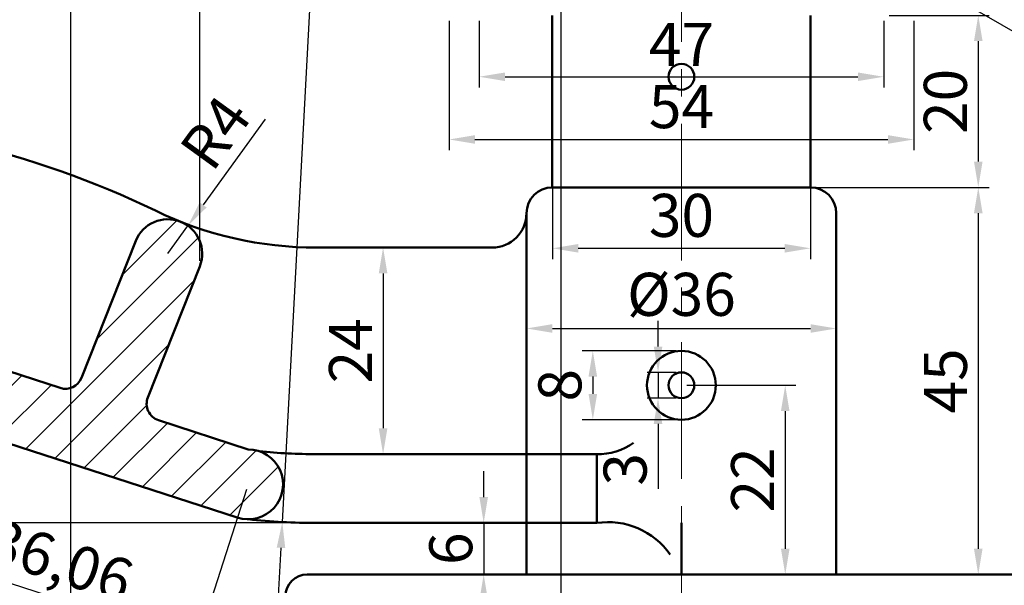
# Model space of a CAD drawing. Units: millimetres. Extents: x 98 to 674, y 38 to 476.
# Tile 3 of 7: x 200 to 315, y 131 to 197. Entities that reach past the tile are written whole.
import ezdxf

# ---------------------------------------------------------------- set-up
doc = ezdxf.new("R2010")
doc.units = ezdxf.units.MM
doc.header["$LTSCALE"] = 0.5
doc.linetypes.add('CENTER', pattern=[50.8, 31.75, -6.35, 6.35, -6.35])
for name, color, linetype, lineweight in [('M-CNTR', 1, 'CENTER', 18), ('M-DIMS', 2, 'Continuous', 25), ('M-HATC', 8, 'Continuous', 18), ('M-OUTL', 7, 'Continuous', 50)]:
    doc.layers.add(name, color=color, linetype=linetype, lineweight=lineweight)
doc.styles.get("Standard").update_dxf_attribs({"font": 'arial.ttf'})
doc.dimstyles.new('ISO-25', dxfattribs={"dimtxt": 5, "dimasz": 3, "dimexe": 1.25, "dimexo": 0.625, "dimtad": 1, "dimtxsty": 'Standard', "dimcen": 2.5, "dimadec": 0, "dimazin": 0, "dimtfac": 1, "dimtmove": 0, "dimatfit": 3, "dimfxl": 1, "dimarcsym": 0})

# ---------------------------------------------------------------- blocks, each defined once
blk = doc.blocks.new('*D21')
at = {"layer": 'Defpoints', "color": 0, "ltscale": 0.5, "transparency": 16777216}
for p in [(327.04, 262.55), (348.82, 249.98), (295.37, 207.69)]:
    blk.add_point(p, dxfattribs=at)
at = {"layer": 'M-DIMS', "color": 0, "lineweight": -2, "ltscale": 0.5, "transparency": 16777216}
for p, q in [((327.58, 262.24), (349.9, 249.35)), ((318.64, 197.71), (347.32, 247.38)), ((295.91, 207.37), (318.22, 194.49))]:
    blk.add_line(p, q, dxfattribs=at)
at = {"layer": 'M-DIMS', "color": 0, "ltscale": 0.5, "transparency": 16777216}
for points in [[(346.89, 247.63), (347.75, 247.13), (348.82, 249.98)], [(318.21, 197.96), (319.08, 197.46), (317.14, 195.11)]]:
    blk.add_solid(points, dxfattribs=at)
at = {"layer": 'M-DIMS', "color": 0, "ltscale": 0.5, "transparency": 16777216, "insert": (329.84, 224.36), "char_height": 5, "attachment_point": 5, "rotation": 60}
blk.add_mtext('63,35', dxfattribs=at)
blk = doc.blocks.new('*D29')
at = {"layer": 'Defpoints', "color": 0, "ltscale": 0.5, "transparency": 16777216}
for p in [(253.87, 197.69), (300.87, 197.69), (300.87, 190.55)]:
    blk.add_point(p, dxfattribs=at)
at = {"layer": 'M-DIMS', "color": 0, "lineweight": -2, "ltscale": 0.5, "transparency": 16777216}
for p, q in [((253.87, 197.06), (253.87, 189.3)), ((300.87, 197.06), (300.87, 189.3)), ((256.87, 190.55), (297.87, 190.55))]:
    blk.add_line(p, q, dxfattribs=at)
at = {"layer": 'M-DIMS', "color": 0, "ltscale": 0.5, "transparency": 16777216}
for points in [[(256.87, 191.05), (256.87, 190.05), (253.87, 190.55)], [(297.87, 191.05), (297.87, 190.05), (300.87, 190.55)]]:
    blk.add_solid(points, dxfattribs=at)
at = {"layer": 'M-DIMS', "color": 0, "ltscale": 0.5, "transparency": 16777216, "insert": (277.37, 193.67), "char_height": 5, "attachment_point": 5}
blk.add_mtext('47', dxfattribs=at)
blk = doc.blocks.new('*D30')
at = {"layer": 'Defpoints', "color": 0, "ltscale": 0.5, "transparency": 16777216}
for p in [(250.37, 197.69), (304.37, 197.69), (304.37, 183.26)]:
    blk.add_point(p, dxfattribs=at)
at = {"layer": 'M-DIMS', "color": 0, "lineweight": -2, "ltscale": 0.5, "transparency": 16777216}
for p, q in [((250.37, 197.06), (250.37, 182.01)), ((304.37, 197.06), (304.37, 182.01)), ((253.37, 183.26), (301.37, 183.26))]:
    blk.add_line(p, q, dxfattribs=at)
at = {"layer": 'M-DIMS', "color": 0, "ltscale": 0.5, "transparency": 16777216}
for points in [[(253.37, 183.76), (253.37, 182.76), (250.37, 183.26)], [(301.37, 183.76), (301.37, 182.76), (304.37, 183.26)]]:
    blk.add_solid(points, dxfattribs=at)
at = {"layer": 'M-DIMS', "color": 0, "ltscale": 0.5, "transparency": 16777216, "insert": (277.37, 186.43), "char_height": 5, "attachment_point": 5}
blk.add_mtext('54', dxfattribs=at)
blk = doc.blocks.new('*D31')
at = {"layer": 'Defpoints', "color": 0, "ltscale": 0.5, "transparency": 16777216}
for p in [(262.37, 179.48), (292.37, 179.48), (292.37, 170.61)]:
    blk.add_point(p, dxfattribs=at)
at = {"layer": 'M-DIMS', "color": 0, "lineweight": -2, "ltscale": 0.5, "transparency": 16777216}
for p, q in [((262.37, 178.85), (262.37, 169.36)), ((292.37, 178.85), (292.37, 169.36)), ((265.37, 170.61), (289.37, 170.61))]:
    blk.add_line(p, q, dxfattribs=at)
at = {"layer": 'M-DIMS', "color": 0, "ltscale": 0.5, "transparency": 16777216}
for points in [[(265.37, 171.11), (265.37, 170.11), (262.37, 170.61)], [(289.37, 171.11), (289.37, 170.11), (292.37, 170.61)]]:
    blk.add_solid(points, dxfattribs=at)
at = {"layer": 'M-DIMS', "color": 0, "ltscale": 0.5, "transparency": 16777216, "insert": (277.37, 173.79), "char_height": 5, "attachment_point": 5}
blk.add_mtext('30', dxfattribs=at)
blk = doc.blocks.new('*D32')
at = {"layer": 'Defpoints', "color": 0, "ltscale": 0.5, "transparency": 16777216}
for p in [(259.37, 161.17), (295.37, 161.29), (295.37, 161.17)]:
    blk.add_point(p, dxfattribs=at)
at = {"layer": 'M-DIMS', "color": 0, "lineweight": -2, "ltscale": 0.5, "transparency": 16777216}
for p, q in [((259.37, 161.79), (259.37, 162.54)), ((295.37, 161.79), (295.37, 162.54)), ((262.37, 161.29), (292.37, 161.29))]:
    blk.add_line(p, q, dxfattribs=at)
at = {"layer": 'M-DIMS', "color": 0, "ltscale": 0.5, "transparency": 16777216}
for points in [[(262.37, 161.79), (262.37, 160.79), (259.37, 161.29)], [(292.37, 161.79), (292.37, 160.79), (295.37, 161.29)]]:
    blk.add_solid(points, dxfattribs=at)
at = {"layer": 'M-DIMS', "color": 0, "ltscale": 0.5, "transparency": 16777216, "insert": (277.37, 164.61), "char_height": 5, "attachment_point": 5}
blk.add_mtext('%%C36', dxfattribs=at)
blk = doc.blocks.new('*D33')
at = {"layer": 'Defpoints', "color": 0, "ltscale": 0.5, "transparency": 16777216}
for p in [(300.87, 197.69), (292.37, 177.69), (311.86, 177.69)]:
    blk.add_point(p, dxfattribs=at)
at = {"layer": 'M-DIMS', "color": 0, "lineweight": -2, "ltscale": 0.5, "transparency": 16777216}
for p, q in [((301.49, 197.69), (313.11, 197.69)), ((311.86, 194.69), (311.86, 180.69)), ((292.99, 177.69), (313.11, 177.69))]:
    blk.add_line(p, q, dxfattribs=at)
at = {"layer": 'M-DIMS', "color": 0, "ltscale": 0.5, "transparency": 16777216}
for points in [[(311.36, 194.69), (312.36, 194.69), (311.86, 197.69)], [(311.36, 180.69), (312.36, 180.69), (311.86, 177.69)]]:
    blk.add_solid(points, dxfattribs=at)
at = {"layer": 'M-DIMS', "color": 0, "ltscale": 0.5, "transparency": 16777216, "insert": (308.68, 187.69), "char_height": 5, "attachment_point": 5, "rotation": 90}
blk.add_mtext('20', dxfattribs=at)
blk = doc.blocks.new('*D34')
at = {"layer": 'Defpoints', "color": 0, "ltscale": 0.5, "transparency": 16777216}
for p in [(303.05, 177.69), (303.05, 132.69), (311.86, 132.69)]:
    blk.add_point(p, dxfattribs=at)
at = {"layer": 'M-DIMS', "color": 0, "lineweight": -2, "ltscale": 0.5, "transparency": 16777216}
for p, q in [((303.68, 177.69), (313.11, 177.69)), ((311.86, 174.69), (311.86, 135.69)), ((303.68, 132.69), (313.11, 132.69))]:
    blk.add_line(p, q, dxfattribs=at)
at = {"layer": 'M-DIMS', "color": 0, "ltscale": 0.5, "transparency": 16777216}
for points in [[(311.36, 174.69), (312.36, 174.69), (311.86, 177.69)], [(311.36, 135.69), (312.36, 135.69), (311.86, 132.69)]]:
    blk.add_solid(points, dxfattribs=at)
at = {"layer": 'M-DIMS', "color": 0, "ltscale": 0.5, "transparency": 16777216, "insert": (308.69, 155.19), "char_height": 5, "attachment_point": 5, "rotation": 90}
blk.add_mtext('45', dxfattribs=at)
blk = doc.blocks.new('*D35')
at = {"layer": 'Defpoints', "color": 0, "ltscale": 0.5, "transparency": 16777216}
for p in [(277.37, 154.69), (277.37, 132.69), (289.43, 132.69)]:
    blk.add_point(p, dxfattribs=at)
at = {"layer": 'M-DIMS', "color": 0, "lineweight": -2, "ltscale": 0.5, "transparency": 16777216}
for p, q in [((277.99, 154.69), (290.68, 154.69)), ((289.43, 151.69), (289.43, 135.69)), ((277.99, 132.69), (290.68, 132.69))]:
    blk.add_line(p, q, dxfattribs=at)
at = {"layer": 'M-DIMS', "color": 0, "ltscale": 0.5, "transparency": 16777216}
for points in [[(288.93, 151.69), (289.93, 151.69), (289.43, 154.69)], [(288.93, 135.69), (289.93, 135.69), (289.43, 132.69)]]:
    blk.add_solid(points, dxfattribs=at)
at = {"layer": 'M-DIMS', "color": 0, "ltscale": 0.5, "transparency": 16777216, "insert": (286.29, 143.69), "char_height": 5, "attachment_point": 5, "rotation": 90}
blk.add_mtext('22', dxfattribs=at)
blk = doc.blocks.new('*D36')
at = {"layer": 'Defpoints', "color": 0, "ltscale": 0.5, "transparency": 16777216}
for p in [(277.37, 156.19), (274.65, 153.19), (277.37, 153.19)]:
    blk.add_point(p, dxfattribs=at)
at = {"layer": 'M-DIMS', "color": 0, "lineweight": -2, "ltscale": 0.5, "transparency": 16777216}
for p, q in [((274.65, 159.19), (274.65, 162.19)), ((276.74, 156.19), (273.4, 156.19)), ((274.65, 156.19), (274.65, 153.19)), ((276.74, 153.19), (273.4, 153.19)), ((274.65, 150.19), (274.65, 142.66))]:
    blk.add_line(p, q, dxfattribs=at)
at = {"layer": 'M-DIMS', "color": 0, "ltscale": 0.5, "transparency": 16777216}
for points in [[(274.15, 159.19), (275.15, 159.19), (274.65, 156.19)], [(274.15, 150.19), (275.15, 150.19), (274.65, 153.19)]]:
    blk.add_solid(points, dxfattribs=at)
at = {"layer": 'M-DIMS', "color": 0, "ltscale": 0.5, "transparency": 16777216, "insert": (271.47, 144.92), "char_height": 5, "attachment_point": 5, "rotation": 90}
blk.add_mtext('3', dxfattribs=at)
blk = doc.blocks.new('*D37')
at = {"layer": 'Defpoints', "color": 0, "ltscale": 0.5, "transparency": 16777216}
for p in [(277.37, 158.69), (267.07, 150.69), (277.37, 150.69)]:
    blk.add_point(p, dxfattribs=at)
at = {"layer": 'M-DIMS', "color": 0, "lineweight": -2, "ltscale": 0.5, "transparency": 16777216}
for p, q in [((276.74, 158.69), (265.82, 158.69)), ((267.07, 155.69), (267.07, 153.69)), ((276.74, 150.69), (265.82, 150.69))]:
    blk.add_line(p, q, dxfattribs=at)
at = {"layer": 'M-DIMS', "color": 0, "ltscale": 0.5, "transparency": 16777216}
for points in [[(266.57, 155.69), (267.57, 155.69), (267.07, 158.69)], [(266.57, 153.69), (267.57, 153.69), (267.07, 150.69)]]:
    blk.add_solid(points, dxfattribs=at)
at = {"layer": 'M-DIMS', "color": 0, "ltscale": 0.5, "transparency": 16777216, "insert": (263.89, 154.69), "char_height": 5, "attachment_point": 5, "rotation": 90}
blk.add_mtext('8', dxfattribs=at)
blk = doc.blocks.new('*D38')
at = {"layer": 'Defpoints', "color": 0, "ltscale": 0.5, "transparency": 16777216}
for p in [(254.39, 138.69), (254.39, 132.69), (254.39, 132.69)]:
    blk.add_point(p, dxfattribs=at)
at = {"layer": 'M-DIMS', "color": 0, "lineweight": -2, "ltscale": 0.5, "transparency": 16777216}
for p, q in [((254.39, 141.69), (254.39, 144.69)), ((254.39, 138.69), (254.39, 132.69)), ((255.02, 138.69), (255.64, 138.69)), ((255.02, 132.69), (255.64, 132.69)), ((254.39, 129.69), (254.39, 126.69))]:
    blk.add_line(p, q, dxfattribs=at)
at = {"layer": 'M-DIMS', "color": 0, "ltscale": 0.5, "transparency": 16777216}
for points in [[(253.89, 141.69), (254.89, 141.69), (254.39, 138.69)], [(253.89, 129.69), (254.89, 129.69), (254.39, 132.69)]]:
    blk.add_solid(points, dxfattribs=at)
at = {"layer": 'M-DIMS', "color": 0, "ltscale": 0.5, "transparency": 16777216, "insert": (251.21, 135.69), "char_height": 5, "attachment_point": 5, "rotation": 90}
blk.add_mtext('6', dxfattribs=at)
blk = doc.blocks.new('*D50')
at = {"layer": 'Defpoints', "color": 0, "ltscale": 0.5, "transparency": 16777216}
for p in [(149.37, 153.69), (149.37, 113.28), (277.37, 112.69)]:
    blk.add_point(p, dxfattribs=at)
at = {"layer": 'M-DIMS', "color": 0, "lineweight": -2, "ltscale": 0.5, "transparency": 16777216}
for p, q in [((149.37, 153.06), (149.37, 112.03)), ((277.37, 113.31), (277.37, 114.53)), ((274.37, 113.28), (152.37, 113.28))]:
    blk.add_line(p, q, dxfattribs=at)
at = {"layer": 'M-DIMS', "color": 0, "ltscale": 0.5, "transparency": 16777216}
for points in [[(152.37, 113.78), (152.37, 112.78), (149.37, 113.28)], [(274.37, 113.78), (274.37, 112.78), (277.37, 113.28)]]:
    blk.add_solid(points, dxfattribs=at)
at = {"layer": 'M-DIMS', "color": 0, "ltscale": 0.5, "transparency": 16777216, "insert": (213.37, 116.46), "char_height": 5, "attachment_point": 5}
blk.add_mtext('128', dxfattribs=at)
blk = doc.blocks.new('*D52')
at = {"layer": 'Defpoints', "color": 0, "ltscale": 0.5, "transparency": 16777216}
for p in [(135.65, 153.69), (149.37, 153.69), (251.25, 138.69)]:
    blk.add_point(p, dxfattribs=at)
at = {"layer": 'M-DIMS', "color": 0, "lineweight": -2, "ltscale": 0.5, "transparency": 16777216}
for p, q in [((148.74, 153.69), (134.4, 153.69)), ((135.65, 141.69), (135.65, 150.69)), ((250.63, 138.69), (134.4, 138.69))]:
    blk.add_line(p, q, dxfattribs=at)
at = {"layer": 'M-DIMS', "color": 0, "ltscale": 0.5, "transparency": 16777216}
for points in [[(135.15, 150.69), (136.15, 150.69), (135.65, 153.69)], [(135.15, 141.69), (136.15, 141.69), (135.65, 138.69)]]:
    blk.add_solid(points, dxfattribs=at)
at = {"layer": 'M-DIMS', "color": 0, "ltscale": 0.5, "transparency": 16777216, "insert": (132.47, 146.19), "char_height": 5, "attachment_point": 5, "rotation": 90}
blk.add_mtext('15', dxfattribs=at)
blk = doc.blocks.new('*D53')
at = {"layer": 'Defpoints', "color": 0, "ltscale": 0.5, "transparency": 16777216}
for p in [(192.69, 154.23), (227.02, 143.17), (221.06, 124.69)]:
    blk.add_point(p, dxfattribs=at)
at = {"layer": 'M-DIMS', "color": 0, "lineweight": -2, "ltscale": 0.5, "transparency": 16777216}
for p, q in [((192.5, 153.64), (186.35, 134.56)), ((226.82, 142.58), (220.68, 123.5)), ((189.59, 134.83), (218.21, 125.61))]:
    blk.add_line(p, q, dxfattribs=at)
at = {"layer": 'M-DIMS', "color": 0, "ltscale": 0.5, "transparency": 16777216}
for points in [[(189.75, 135.31), (189.44, 134.36), (186.74, 135.75)], [(218.36, 126.09), (218.05, 125.14), (221.06, 124.69)]]:
    blk.add_solid(points, dxfattribs=at)
at = {"layer": 'M-DIMS', "color": 0, "ltscale": 0.5, "transparency": 16777216, "insert": (205.01, 133.68), "char_height": 5, "attachment_point": 5, "rotation": 342.137}
blk.add_mtext('36,06', dxfattribs=at)
blk = doc.blocks.new('*D54')
at = {"layer": 'Defpoints', "color": 0, "ltscale": 0.5, "transparency": 16777216}
for p in [(245.17, 170.69), (242.7, 146.69), (245.17, 146.69)]:
    blk.add_point(p, dxfattribs=at)
at = {"layer": 'M-DIMS', "color": 0, "lineweight": -2, "ltscale": 0.5, "transparency": 16777216}
for p, q in [((244.55, 170.69), (241.45, 170.69)), ((242.7, 167.69), (242.7, 149.69)), ((244.55, 146.69), (241.45, 146.69))]:
    blk.add_line(p, q, dxfattribs=at)
at = {"layer": 'M-DIMS', "color": 0, "ltscale": 0.5, "transparency": 16777216}
for points in [[(242.2, 167.69), (243.2, 167.69), (242.7, 170.69)], [(242.2, 149.69), (243.2, 149.69), (242.7, 146.69)]]:
    blk.add_solid(points, dxfattribs=at)
at = {"layer": 'M-DIMS', "color": 0, "ltscale": 0.5, "transparency": 16777216, "insert": (239.56, 158.69), "char_height": 5, "attachment_point": 5, "rotation": 90}
blk.add_mtext('24', dxfattribs=at)
blk = doc.blocks.new('*D68')
at = {"layer": 'Defpoints', "color": 0, "ltscale": 0.5, "transparency": 16777216}
for p in [(263.37, 325.69), (206.37, 226.96), (263.37, 42.76)]:
    blk.add_point(p, dxfattribs=at)
at = {"layer": 'M-DIMS', "color": 0, "lineweight": -2, "ltscale": 0.5, "transparency": 16777216}
for p, q in [((263.37, 325.06), (263.37, 41.51)), ((206.37, 226.33), (206.37, 41.51)), ((209.37, 42.76), (260.37, 42.76))]:
    blk.add_line(p, q, dxfattribs=at)
at = {"layer": 'M-DIMS', "color": 0, "ltscale": 0.5, "transparency": 16777216}
for points in [[(209.37, 43.26), (209.37, 42.26), (206.37, 42.76)], [(260.37, 43.26), (260.37, 42.26), (263.37, 42.76)]]:
    blk.add_solid(points, dxfattribs=at)
at = {"layer": 'M-DIMS', "color": 0, "ltscale": 0.5, "transparency": 16777216, "insert": (234.87, 45.93), "char_height": 5, "attachment_point": 5}
blk.add_mtext('57', dxfattribs=at)
blk = doc.blocks.new('*D71')
at = {"layer": 'Defpoints', "color": 0, "ltscale": 0.5, "transparency": 16777216}
for p in [(269.37, 413.69), (121.37, 76.69), (269.37, 76.69)]:
    blk.add_point(p, dxfattribs=at)
at = {"layer": 'M-DIMS', "color": 0, "lineweight": -2, "ltscale": 0.5, "transparency": 16777216}
for p, q in [((268.74, 413.69), (120.12, 413.69)), ((121.37, 410.69), (121.37, 79.69)), ((268.74, 76.69), (120.12, 76.69))]:
    blk.add_line(p, q, dxfattribs=at)
at = {"layer": 'M-DIMS', "color": 0, "ltscale": 0.5, "transparency": 16777216}
for points in [[(120.87, 410.69), (121.87, 410.69), (121.37, 413.69)], [(120.87, 79.69), (121.87, 79.69), (121.37, 76.69)]]:
    blk.add_solid(points, dxfattribs=at)
at = {"layer": 'M-DIMS', "color": 0, "ltscale": 0.5, "transparency": 16777216, "insert": (118.19, 245.19), "char_height": 5, "attachment_point": 5, "rotation": 90}
blk.add_mtext('337', dxfattribs=at)
blk = doc.blocks.new('*D72')
at = {"layer": 'Defpoints', "color": 0, "ltscale": 0.5, "transparency": 16777216}
for p in [(149.37, 196.69), (323.37, 130.19), (323.37, 42.76)]:
    blk.add_point(p, dxfattribs=at)
at = {"layer": 'M-DIMS', "color": 0, "lineweight": -2, "ltscale": 0.5, "transparency": 16777216}
for p, q in [((149.37, 196.06), (149.37, 41.51)), ((323.37, 129.56), (323.37, 41.51)), ((152.37, 42.76), (320.37, 42.76))]:
    blk.add_line(p, q, dxfattribs=at)
at = {"layer": 'M-DIMS', "color": 0, "ltscale": 0.5, "transparency": 16777216}
for points in [[(152.37, 43.26), (152.37, 42.26), (149.37, 42.76)], [(320.37, 43.26), (320.37, 42.26), (323.37, 42.76)]]:
    blk.add_solid(points, dxfattribs=at)
at = {"layer": 'M-DIMS', "color": 0, "ltscale": 0.5, "transparency": 16777216, "insert": (236.37, 45.9), "char_height": 5, "attachment_point": 5}
blk.add_mtext('174', dxfattribs=at)
blk = doc.blocks.new('*D73')
at = {"layer": 'Defpoints', "color": 0, "ltscale": 0.5, "transparency": 16777216}
for p in [(221.4, 441.69), (221.4, 168.51), (149.37, 153.69)]:
    blk.add_point(p, dxfattribs=at)
at = {"layer": 'M-DIMS', "color": 0, "lineweight": -2, "ltscale": 0.5, "transparency": 16777216}
for p, q in [((149.37, 154.31), (149.37, 442.94)), ((221.4, 169.14), (221.4, 442.94)), ((152.37, 441.69), (218.4, 441.69))]:
    blk.add_line(p, q, dxfattribs=at)
at = {"layer": 'M-DIMS', "color": 0, "ltscale": 0.5, "transparency": 16777216}
for points in [[(152.37, 442.19), (152.37, 441.19), (149.37, 441.69)], [(218.4, 442.19), (218.4, 441.19), (221.4, 441.69)]]:
    blk.add_solid(points, dxfattribs=at)
at = {"layer": 'M-DIMS', "color": 0, "ltscale": 0.5, "transparency": 16777216, "insert": (185.38, 444.87), "char_height": 5, "attachment_point": 5}
blk.add_mtext('72.03', dxfattribs=at)
blk = doc.blocks.new('*D74')
at = {"layer": 'Defpoints', "color": 0, "ltscale": 0.5, "transparency": 16777216}
for p in [(220.03, 173.23), (217.68, 169.99)]:
    blk.add_point(p, dxfattribs=at)
at = {"layer": 'M-DIMS', "color": 0, "lineweight": -2, "ltscale": 0.5, "transparency": 16777216}
for p, q in [((228.99, 185.61), (221.79, 175.66)), ((217.68, 169.99), (220.03, 173.23))]:
    blk.add_line(p, q, dxfattribs=at)
at = {"layer": 'M-DIMS', "color": 0, "ltscale": 0.5, "transparency": 16777216}
blk.add_solid([(221.38, 175.95), (222.19, 175.36), (220.03, 173.23)], dxfattribs=at)
at = {"layer": 'M-DIMS', "color": 0, "ltscale": 0.5, "transparency": 16777216, "insert": (223.74, 183.68), "char_height": 5, "attachment_point": 5, "rotation": 54.0979}
blk.add_mtext('R4', dxfattribs=at)
blk = doc.blocks.new('*D76')
at = {"layer": 'Defpoints', "color": 0, "ltscale": 0.5, "transparency": 16777216}
for p in [(234.98, 213.69), (230.99, 138.79)]:
    blk.add_point(p, dxfattribs=at)
at = {"layer": 'M-DIMS', "color": 0, "lineweight": -2, "ltscale": 0.5, "transparency": 16777216}
for p, q in [((234.98, 213.69), (230.99, 138.79)), ((228.25, 87.25), (230.84, 135.8))]:
    blk.add_line(p, q, dxfattribs=at)
at = {"layer": 'M-DIMS', "color": 0, "ltscale": 0.5, "transparency": 16777216}
blk.add_solid([(230.34, 135.82), (231.33, 135.77), (230.99, 138.79)], dxfattribs=at)
at = {"layer": 'M-DIMS', "color": 0, "ltscale": 0.5, "transparency": 16777216, "insert": (225.44, 94.02), "char_height": 5, "attachment_point": 5, "rotation": 86.9505}
blk.add_mtext('R75', dxfattribs=at)
blk = doc.blocks.new('*D78')
at = {"layer": 'Defpoints', "color": 0, "ltscale": 0.5, "transparency": 16777216}
for p in [(291.37, 325.69), (348.37, 226.96)]:
    blk.add_point(p, dxfattribs=at)
at = {"layer": 'M-DIMS', "color": 0, "lineweight": -2, "ltscale": 0.5, "transparency": 16777216}
for p, q in [((291.37, 325.69), (348.37, 226.96)), ((386.83, 160.33), (349.87, 224.36))]:
    blk.add_line(p, q, dxfattribs=at)
at = {"layer": 'M-DIMS', "color": 0, "ltscale": 0.5, "transparency": 16777216}
blk.add_solid([(350.3, 224.61), (349.43, 224.11), (348.37, 226.96)], dxfattribs=at)
at = {"layer": 'M-DIMS', "color": 0, "ltscale": 0.5, "transparency": 16777216, "insert": (385.28, 169.29), "char_height": 5, "attachment_point": 5, "rotation": 300.0001}
blk.add_mtext('R114', dxfattribs=at)

msp = doc.modelspace()

# ---------------------------------------------------------------- hatches: boundary and pattern name
at = {"layer": 'M-HATC', "ltscale": 0.5}
h = msp.add_hatch(dxfattribs=at)
h.set_pattern_fill('ANSI31', color=256)
h.paths.add_polyline_path([(215.3645, 153.2734), (221.3997, 168.5142, 1), (213.9617, 171.4596), (207.6565, 155.5371, -0.39645231), (205.1754, 154.3725), (194.5293, 157.8537, 1), (190.8572, 150.6104, -0.00464805), (192.1907, 150.2028), (225.763, 139.3083, 1.17062936), (227.0163, 147.2309), (216.6024, 150.6361, -0.43220072)])

# ---------------------------------------------------------------- linework, layer by layer
at = {"layer": 'M-CNTR'}
msp.add_line((277.365, 413.6855), (277.365, 70.7639), dxfattribs=at)
at = {"layer": 'M-OUTL'}
for p, q in [((262.365, 197.6855), (262.365, 177.6855)), ((292.365, 177.6855), (292.365, 197.6855)), ((262.365, 177.6855), (292.365, 177.6855)), ((262.365, 177.6855), (292.365, 177.6855)), ((259.365, 132.6855), (259.365, 174.6855)), ((295.365, 174.6855), (295.365, 132.6855)), ((267.5202, 146.6855), (234.9849, 146.6855)), ((267.5202, 138.6855), (234.9849, 138.6855)), ((295.365, 132.6855), (259.365, 132.6855))]:
    msp.add_line(p, q, dxfattribs=at)
at = {"layer": 'M-OUTL', "ltscale": 0.5}
for p, q in [((207.6565, 155.5371), (213.9617, 171.4596)), ((215.3645, 153.2734), (221.3997, 168.5142)), ((194.5293, 157.8537), (205.1754, 154.3725)), ((192.1907, 150.2028), (225.763, 139.3083)), ((216.6024, 150.6361), (227.0163, 147.2309)), ((267.5202, 146.6855), (267.5202, 138.6855)), ((277.365, 132.6855), (277.365, 138.6855))]:
    msp.add_line(p, q, dxfattribs=at)
at = {"layer": 'M-OUTL'}
msp.add_lwpolyline([(259.365, 174.6855), (259.365, 174.6855, -0.41421356), (255.365, 170.6855), (234.9849, 170.6855, -0.11323701), (216.2416, 174.9855, 0.11151094), (170.3309, 185.683, -0.41221797), (165.365, 190.6829), (165.365, 196.6855)], format="xyb", dxfattribs=at)
msp.add_lwpolyline([(320.865, 132.6855), (233.865, 132.6855, 1), (233.865, 127.6855), (320.865, 127.6855, 1)], format="xyb", close=True, dxfattribs=at)
at = {"layer": 'M-OUTL', "ltscale": 0.5}
msp.add_circle((277.365, 190.5497), 1.5, dxfattribs=at)
at = {"layer": 'M-OUTL'}
for radius in [4, 1.5]:
    msp.add_circle((277.365, 154.6855), radius, dxfattribs=at)
for centre, radius, start, end in [((262.365, 174.6855), 3, 90, 180), ((292.365, 174.6855), 3, 0, 90), ((234.9849, 213.6855), 67, 264.284271, 270), ((234.9849, 213.6855), 75, 263.900929, 270)]:
    msp.add_arc(centre, radius, start, end, dxfattribs=at)
at = {"layer": 'M-OUTL', "ltscale": 0.5}
for centre, radius, start, end in [((217.6807, 169.9869), 4, 338.396932, 158.396932), ((205.797, 156.2735), 2, 251.893074, 338.396932), ((217.224, 152.537), 2, 158.396932, 251.893074), ((267.6667, 153.9397), 7.2557, 268.843493, 304.869517), ((227.0163, 143.1705), 4.0605, 252.021289, 90), ((268.8247, 129.959), 8.8234, 34.895768, 98.502029)]:
    msp.add_arc(centre, radius, start, end, dxfattribs=at)

# ---------------------------------------------------------------- dimensions: what is measured, and where the dimension line sits
at = {"layer": 'M-DIMS', "ltscale": 0.5}
for base, p1, p2, override, picture, middle in [((221.3997, 441.6855), (149.365, 153.6855), (221.3997, 168.5142), {"dimdec": 2, "dimlfac": 1, "dimrnd": 0, "dimzin": 0, "dimdsep": 46, "dimlunit": 2}, '*D73', (185.3824, 444.8651)), ((263.365, 42.7639), (206.365, 226.9586), (263.365, 325.6855), {"dimdec": 0, "dimlfac": 1, "dimrnd": 0, "dimzin": 0, "dimdsep": 46, "dimlunit": 2}, '*D68', (234.865, 45.9316)), ((304.365, 183.2593), (250.365, 197.6855), (304.365, 197.6855), {"dimclrd": 0, "dimclre": 0, "dimclrt": 0}, '*D30', (277.365, 186.4269)), ((300.865, 190.5497), (253.865, 197.6855), (300.865, 197.6855), {"dimclrd": 0, "dimclre": 0, "dimclrt": 0}, '*D29', (277.365, 193.6747)), ((323.365, 42.7639), (149.365, 196.6855), (323.365, 130.1855), {"dimdec": 0, "dimlfac": 1, "dimrnd": 0, "dimzin": 0, "dimdsep": 46, "dimlunit": 2}, '*D72', (236.365, 45.8992)), ((292.365, 170.6148), (262.365, 179.4762), (292.365, 179.4762), {"dimclrd": 0, "dimclre": 0, "dimclrt": 0}, '*D31', (277.365, 173.7944)), ((149.365, 113.2817), (277.365, 112.6855), (149.365, 153.6855), {"dimclrd": 0, "dimclre": 0, "dimclrt": 0}, '*D50', (213.365, 116.4596))]:
    dim = msp.add_linear_dim(base=base, p1=p1, p2=p2, dimstyle='ISO-25', override=override, dxfattribs=at)
    dim.commit()
    dim.dimension.update_dxf_attribs({"geometry": picture, "text_midpoint": middle})
for base, p1, p2, override, picture, middle in [((121.365, 76.6855), (269.365, 413.6855), (269.365, 76.6855), {"dimdec": 0, "dimlfac": 1, "dimrnd": 0, "dimzin": 0, "dimdsep": 46, "dimlunit": 2}, '*D71', (118.1855, 245.1855)), ((311.8607, 177.6855), (300.865, 197.6855), (292.365, 177.6855), {"dimclrd": 0, "dimclre": 0, "dimclrt": 0}, '*D33', (308.6828, 187.6855)), ((311.8607, 132.6855), (303.0504, 177.6855), (303.0504, 132.6855), {"dimclrd": 0, "dimclre": 0, "dimclrt": 0}, '*D34', (308.6931, 155.1855)), ((274.6545, 153.1855), (277.365, 156.1855), (277.365, 153.1855), {"dimclrd": 0, "dimclre": 0, "dimclrt": 0}, '*D36', (271.475, 144.9234)), ((267.0703, 150.6855), (277.365, 158.6855), (277.365, 150.6855), {"dimclrd": 0, "dimclre": 0, "dimclrt": 0}, '*D37', (263.8924, 154.6855)), ((289.426, 132.6855), (277.365, 154.6855), (277.365, 132.6855), {"dimclrd": 0, "dimclre": 0, "dimclrt": 0}, '*D35', (286.2908, 143.6855)), ((135.6524, 153.6855), (251.2525, 138.6855), (149.365, 153.6855), {"dimclrd": 0, "dimclre": 0, "dimclrt": 0}, '*D52', (132.4745, 146.1855)), ((254.3923, 132.6855), (254.3923, 138.6855), (254.3923, 132.6855), {"dimclrd": 0, "dimclre": 0, "dimclrt": 0}, '*D38', (251.2145, 135.6855))]:
    dim = msp.add_linear_dim(base=base, p1=p1, p2=p2, angle=90, dimstyle='ISO-25', override=override, dxfattribs=at)
    dim.commit()
    dim.dimension.update_dxf_attribs({"geometry": picture, "text_midpoint": middle})
for center, mpoint, picture, middle in [((291.365, 325.6855), (348.3652, 226.9587), '*D78', (382.5653, 167.7226)), ((234.9849, 213.6855), (230.995, 138.7917), '*D76', (228.601, 93.8554))]:
    dim = msp.add_radius_dim(center=center, mpoint=mpoint, dimstyle='ISO-25', override={"dimdec": 0, "dimlfac": 1, "dimrnd": 0, "dimzin": 0, "dimdsep": 46, "dimlunit": 2}, dxfattribs=at)
    dim.commit()
    dim.dimension.update_dxf_attribs({"geometry": picture, "text_midpoint": middle, "dimtype": 164})
for p1, p2, distance, picture, middle in [((295.365, 207.6855), (327.0419, 262.5515), -25.146, '*D21', (329.8371, 224.3604)), ((245.175, 170.6855), (245.175, 146.6855), -2.4781, '*D54', (239.5617, 158.6855)), ((192.6933, 154.232), (227.0163, 143.1705), -19.4157, '*D53', (205.0126, 133.6763))]:
    dim = msp.add_aligned_dim(p1=p1, p2=p2, distance=distance, dimstyle='ISO-25', override={"dimclrd": 0, "dimclre": 0, "dimclrt": 0}, dxfattribs=at)
    dim.commit()
    dim.dimension.update_dxf_attribs({"geometry": picture, "text_midpoint": middle})
dim = msp.add_radius_dim(center=(217.6807, 169.9869), mpoint=(220.0263, 173.227), dimstyle='ISO-25', override={"dimdec": 0, "dimlfac": 1, "dimrnd": 0, "dimzin": 0, "dimdsep": 46, "dimlunit": 2}, dxfattribs=at)
dim.commit()
dim.dimension.update_dxf_attribs({"geometry": '*D74', "text_midpoint": (223.7379, 183.6831)})
dim = msp.add_linear_dim(base=(295.365, 161.2882), p1=(259.365, 161.1697), p2=(295.365, 161.1697), text='%%C<>', dimstyle='ISO-25', override={"dimclrd": 0, "dimclre": 0, "dimclrt": 0}, dxfattribs=at)
dim.commit()
dim.dimension.update_dxf_attribs({"geometry": '*D32', "text_midpoint": (277.365, 164.6059)})

doc.saveas('drawing.dxf')
